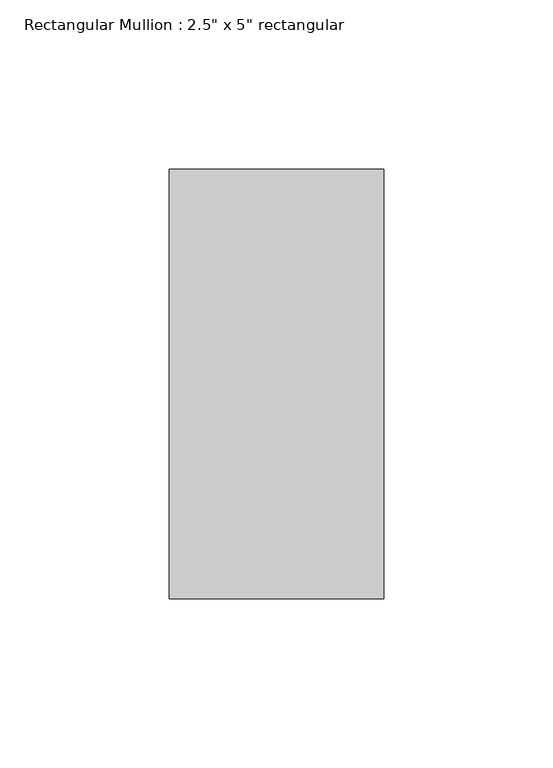
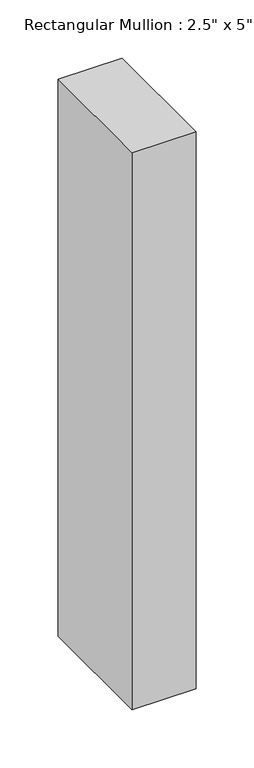
"""IFC4 building model written with IfcOpenShell, lengths in millimetres: member geometry."""

from ifc_helpers import new_model, si_unit, frame, origin, place, context, project, spatial, polyline, outline, extrude, source, transform, mapped, element, save


def member_623bfa76(model_context):
    return source(origin(), model_context, "Body", "SweptSolid", [
        extrude(outline(polyline([(0.0, 63.5), (0.0, -63.5), (-63.5, -63.5), (-63.5, 63.5), (0.0, 63.5)])), frame((0.0, 0.0, -584.2), z_axis=(0.0, 0.0, 1.0), x_axis=(1.0, 0.0, 0.0)), (0.0, 0.0, 1.0), 584.2),
    ])


if __name__ == "__main__":
    model = new_model("IFC4")
    model_context = context("Model", 3, world=origin())
    ifc_project = project(units=[si_unit("LENGTHUNIT", "METRE", prefix="MILLI")], contexts=[model_context])
    site = spatial("IfcSite", under=ifc_project)
    building = spatial("IfcBuilding", under=site)
    placement = place(None, origin())
    member_shape = member_623bfa76(model_context)
    element("IfcMember", 1, ObjectType="Rectangular Mullion : 2.5\" x 5\" rectangular", at=placement, inside=building, context=model_context, shape_type="MappedRepresentation", body=[
        mapped(member_shape, transform((0.0, 0.0, 0.0), x_axis=(1.0, 0.0, 0.0), y_axis=(0.0, 1.0, 0.0), z_axis=(0.0, 0.0, 1.0))),
    ])
    save(model, "model.ifc")

# Revit data of these elements
# Type "Rectangular Mullion : 2.5\" x 5\" rectangular"
#   built-in parameter 1007304 = 0.416667 (stored number, unit not read)
#   built-in parameter 1007301 = 0.104167 (stored number, unit not read)
#   built-in parameter 1007300 = 0.104167 (stored number, unit not read)
# Element 1 (IfcMember, "Rectangular Mullion : 2.5\" x 5\" rectangular")
#   Materials on its faces: "Aluminum"
# Materials
#   "Aluminum": class "Metal", colour RGB 247 247 247, transparency 0, Description = "Aluminum 6061", Cost = 0
